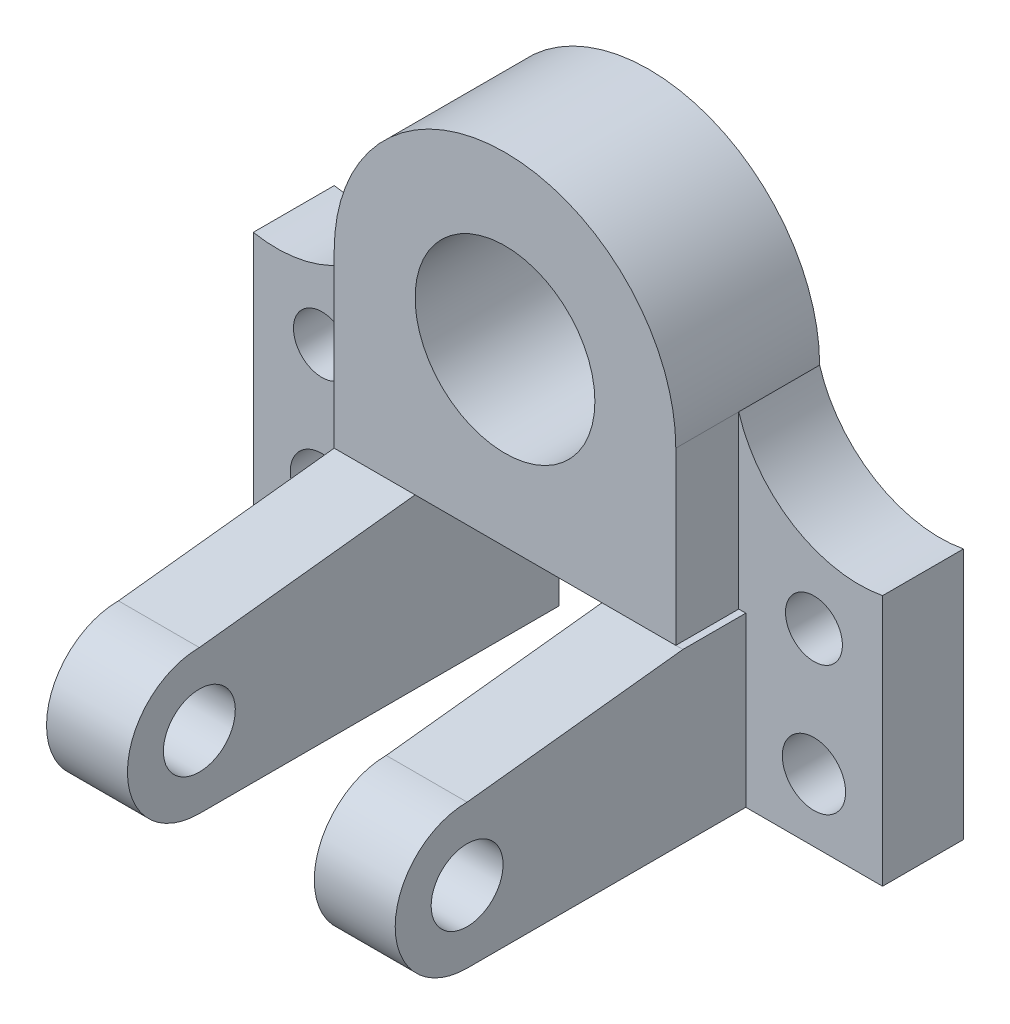
ISO-10303-21;
HEADER;
FILE_DESCRIPTION(('STEP AP214'),'2;1');
FILE_NAME('part.step','',(''),(''),'','','');
FILE_SCHEMA(('AUTOMOTIVE_DESIGN { 1 0 10303 214 1 1 1 1 }'));
ENDSEC;
DATA;
#1=APPLICATION_CONTEXT('core data for automotive mechanical design processes');
#2=APPLICATION_PROTOCOL_DEFINITION('international standard','automotive_design',2000,#1);
#3=PRODUCT_CONTEXT('',#1,'mechanical');
#4=PRODUCT('Part','Part','',(#3));
#5=PRODUCT_RELATED_PRODUCT_CATEGORY('part','',(#4));
#6=PRODUCT_DEFINITION_FORMATION('','',#4);
#7=PRODUCT_DEFINITION_CONTEXT('part definition',#1,'design');
#8=PRODUCT_DEFINITION('design','',#6,#7);
#9=PRODUCT_DEFINITION_SHAPE('','',#8);
#10=(LENGTH_UNIT() NAMED_UNIT(*) SI_UNIT(.MILLI.,.METRE.));
#11=(NAMED_UNIT(*) PLANE_ANGLE_UNIT() SI_UNIT($,.RADIAN.));
#12=(NAMED_UNIT(*) SI_UNIT($,.STERADIAN.) SOLID_ANGLE_UNIT());
#13=UNCERTAINTY_MEASURE_WITH_UNIT(LENGTH_MEASURE(1.E-05),#10,'distance_accuracy_value','');
#14=(GEOMETRIC_REPRESENTATION_CONTEXT(3) GLOBAL_UNCERTAINTY_ASSIGNED_CONTEXT((#13)) GLOBAL_UNIT_ASSIGNED_CONTEXT((#10,
#11,#12)) REPRESENTATION_CONTEXT('',''));
#15=CARTESIAN_POINT('',(0.,0.,0.));
#16=DIRECTION('',(0.,0.,1.));
#17=DIRECTION('',(1.,0.,0.));
#18=AXIS2_PLACEMENT_3D('',#15,#16,#17);
#19=CARTESIAN_POINT('',(-38.,0.,32.));
#20=DIRECTION('',(-1.,0.,0.));
#21=DIRECTION('',(0.,0.,1.));
#22=AXIS2_PLACEMENT_3D('',#19,#20,#21);
#23=PLANE('',#22);
#24=CARTESIAN_POINT('',(-38.,-59.4133546374379,80.));
#25=DIRECTION('',(-1.,0.,0.));
#26=DIRECTION('',(0.,0.,1.));
#27=AXIS2_PLACEMENT_3D('',#24,#25,#26);
#28=CIRCLE('',#27,8.);
#29=CARTESIAN_POINT('',(-38.,-59.4133546374379,88.));
#30=VERTEX_POINT('',#29);
#31=EDGE_CURVE('E434',#30,#30,#28,.T.);
#32=ORIENTED_EDGE('',*,*,#31,.F.);
#33=EDGE_LOOP('',(#32));
#34=FACE_BOUND('',#33,.T.);
#35=DIRECTION('',(0.,0.,-1.));
#36=VECTOR('',#35,1.);
#37=CARTESIAN_POINT('',(-38.,-75.4133546374379,96.));
#38=LINE('',#37,#36);
#39=CARTESIAN_POINT('',(-38.,-75.4133546374379,80.));
#40=VERTEX_POINT('',#39);
#41=CARTESIAN_POINT('',(-38.,-75.4133546374379,18.));
#42=VERTEX_POINT('',#41);
#43=EDGE_CURVE('E230',#40,#42,#38,.T.);
#44=ORIENTED_EDGE('',*,*,#43,.F.);
#45=CARTESIAN_POINT('',(-38.,-59.4133546374379,80.));
#46=DIRECTION('',(-1.,0.,0.));
#47=DIRECTION('',(0.,0.,1.));
#48=AXIS2_PLACEMENT_3D('',#45,#46,#47);
#49=CIRCLE('',#48,16.);
#50=CARTESIAN_POINT('',(-38.,-43.4133546374379,80.));
#51=VERTEX_POINT('',#50);
#52=EDGE_CURVE('E213',#40,#51,#49,.T.);
#53=ORIENTED_EDGE('',*,*,#52,.T.);
#54=DIRECTION('',(0.,0.112067782494009,-0.993700564620387));
#55=VECTOR('',#54,1.);
#56=CARTESIAN_POINT('',(-38.,-33.9591726611396,-3.82985510018196));
#57=LINE('',#56,#55);
#58=CARTESIAN_POINT('',(-38.,-38.,32.));
#59=VERTEX_POINT('',#58);
#60=EDGE_CURVE('E221',#51,#59,#57,.T.);
#61=ORIENTED_EDGE('',*,*,#60,.T.);
#62=DIRECTION('',(0.,1.,0.));
#63=VECTOR('',#62,1.);
#64=CARTESIAN_POINT('',(-38.,0.,32.));
#65=LINE('',#64,#63);
#66=CARTESIAN_POINT('',(-38.,0.,32.));
#67=VERTEX_POINT('',#66);
#68=EDGE_CURVE('E327',#59,#67,#65,.T.);
#69=ORIENTED_EDGE('',*,*,#68,.T.);
#70=DIRECTION('',(0.,0.,-1.));
#71=VECTOR('',#70,1.);
#72=CARTESIAN_POINT('',(-38.,0.,32.));
#73=LINE('',#72,#71);
#74=CARTESIAN_POINT('',(-38.,0.,18.));
#75=VERTEX_POINT('',#74);
#76=EDGE_CURVE('E345',#67,#75,#73,.T.);
#77=ORIENTED_EDGE('',*,*,#76,.T.);
#78=DIRECTION('',(0.,1.,0.));
#79=VECTOR('',#78,1.);
#80=CARTESIAN_POINT('',(-38.,0.,18.));
#81=LINE('',#80,#79);
#82=EDGE_CURVE('E240',#42,#75,#81,.T.);
#83=ORIENTED_EDGE('',*,*,#82,.F.);
#84=EDGE_LOOP('',(#44,#53,#61,#69,#77,#83));
#85=FACE_BOUND('',#84,.T.);
#86=ADVANCED_FACE('F90',(#34,#85),#23,.T.);
#87=CARTESIAN_POINT('',(-20.,-38.,96.));
#88=DIRECTION('',(-1.,0.,0.));
#89=DIRECTION('',(0.,-1.,0.));
#90=AXIS2_PLACEMENT_3D('',#87,#88,#89);
#91=PLANE('',#90);
#92=CARTESIAN_POINT('',(-20.,-59.4133546374379,80.));
#93=DIRECTION('',(-1.,0.,0.));
#94=DIRECTION('',(0.,-1.,0.));
#95=AXIS2_PLACEMENT_3D('',#92,#93,#94);
#96=CIRCLE('',#95,8.);
#97=CARTESIAN_POINT('',(-20.,-67.4133546374379,80.));
#98=VERTEX_POINT('',#97);
#99=EDGE_CURVE('E351',#98,#98,#96,.T.);
#100=ORIENTED_EDGE('',*,*,#99,.T.);
#101=EDGE_LOOP('',(#100));
#102=FACE_BOUND('',#101,.T.);
#103=CARTESIAN_POINT('',(-20.,-59.4133546374379,80.));
#104=DIRECTION('',(-1.,0.,0.));
#105=DIRECTION('',(0.,-1.,0.));
#106=AXIS2_PLACEMENT_3D('',#103,#104,#105);
#107=CIRCLE('',#106,16.);
#108=CARTESIAN_POINT('',(-20.,-75.4133546374379,80.));
#109=VERTEX_POINT('',#108);
#110=CARTESIAN_POINT('',(-20.,-43.4133546374379,80.));
#111=VERTEX_POINT('',#110);
#112=EDGE_CURVE('E350',#109,#111,#107,.T.);
#113=ORIENTED_EDGE('',*,*,#112,.F.);
#114=DIRECTION('',(0.,0.,-1.));
#115=VECTOR('',#114,1.);
#116=CARTESIAN_POINT('',(-20.,-75.4133546374379,96.));
#117=LINE('',#116,#115);
#118=CARTESIAN_POINT('',(-20.,-75.4133546374379,0.));
#119=VERTEX_POINT('',#118);
#120=EDGE_CURVE('E233',#109,#119,#117,.T.);
#121=ORIENTED_EDGE('',*,*,#120,.T.);
#122=DIRECTION('',(0.,1.,0.));
#123=VECTOR('',#122,1.);
#124=CARTESIAN_POINT('',(-20.,-38.,0.));
#125=LINE('',#124,#123);
#126=CARTESIAN_POINT('',(-20.,-38.,0.));
#127=VERTEX_POINT('',#126);
#128=EDGE_CURVE('E385',#119,#127,#125,.T.);
#129=ORIENTED_EDGE('',*,*,#128,.T.);
#130=DIRECTION('',(0.,0.,-1.));
#131=VECTOR('',#130,1.);
#132=CARTESIAN_POINT('',(-20.,-38.,96.));
#133=LINE('',#132,#131);
#134=CARTESIAN_POINT('',(-20.,-38.,32.));
#135=VERTEX_POINT('',#134);
#136=EDGE_CURVE('E244',#135,#127,#133,.T.);
#137=ORIENTED_EDGE('',*,*,#136,.F.);
#138=DIRECTION('',(0.,0.112067782494009,-0.993700564620387));
#139=VECTOR('',#138,1.);
#140=CARTESIAN_POINT('',(-20.,-45.1271563993633,95.19621197612));
#141=LINE('',#140,#139);
#142=EDGE_CURVE('E361',#111,#135,#141,.T.);
#143=ORIENTED_EDGE('',*,*,#142,.F.);
#144=EDGE_LOOP('',(#113,#121,#129,#137,#143));
#145=FACE_BOUND('',#144,.T.);
#146=ADVANCED_FACE('F392',(#102,#145),#91,.F.);
#147=CARTESIAN_POINT('',(39.5715731247638,-38.,96.));
#148=DIRECTION('',(-1.,0.,0.));
#149=DIRECTION('',(0.,0.,1.));
#150=AXIS2_PLACEMENT_3D('',#147,#148,#149);
#151=PLANE('',#150);
#152=CARTESIAN_POINT('',(39.5715731247638,-59.4133546374379,80.));
#153=DIRECTION('',(-1.,0.,0.));
#154=DIRECTION('',(0.,0.,1.));
#155=AXIS2_PLACEMENT_3D('',#152,#153,#154);
#156=CIRCLE('',#155,8.);
#157=CARTESIAN_POINT('',(39.5715731247638,-59.4133546374379,88.));
#158=VERTEX_POINT('',#157);
#159=EDGE_CURVE('E347',#158,#158,#156,.T.);
#160=ORIENTED_EDGE('',*,*,#159,.T.);
#161=EDGE_LOOP('',(#160));
#162=FACE_BOUND('',#161,.T.);
#163=CARTESIAN_POINT('',(39.5715731247638,-59.4133546374379,80.));
#164=DIRECTION('',(-1.,0.,0.));
#165=DIRECTION('',(0.,0.,1.));
#166=AXIS2_PLACEMENT_3D('',#163,#164,#165);
#167=CIRCLE('',#166,16.);
#168=CARTESIAN_POINT('',(39.5715731247638,-75.4133546374379,80.));
#169=VERTEX_POINT('',#168);
#170=CARTESIAN_POINT('',(39.5715731247638,-43.4133546374379,80.));
#171=VERTEX_POINT('',#170);
#172=EDGE_CURVE('E354',#169,#171,#167,.T.);
#173=ORIENTED_EDGE('',*,*,#172,.F.);
#174=DIRECTION('',(0.,0.,-1.));
#175=VECTOR('',#174,1.);
#176=CARTESIAN_POINT('',(39.5715731247638,-75.4133546374379,96.));
#177=LINE('',#176,#175);
#178=CARTESIAN_POINT('',(39.5715731247638,-75.4133546374379,18.));
#179=VERTEX_POINT('',#178);
#180=EDGE_CURVE('E366',#169,#179,#177,.T.);
#181=ORIENTED_EDGE('',*,*,#180,.T.);
#182=DIRECTION('',(0.,-1.,0.));
#183=VECTOR('',#182,1.);
#184=CARTESIAN_POINT('',(39.5715731247638,8.10007584438996,18.));
#185=LINE('',#184,#183);
#186=CARTESIAN_POINT('',(39.5715731247638,-38.,18.));
#187=VERTEX_POINT('',#186);
#188=EDGE_CURVE('E377',#187,#179,#185,.T.);
#189=ORIENTED_EDGE('',*,*,#188,.F.);
#190=DIRECTION('',(0.,0.,-1.));
#191=VECTOR('',#190,1.);
#192=CARTESIAN_POINT('',(39.5715731247638,-38.,96.));
#193=LINE('',#192,#191);
#194=CARTESIAN_POINT('',(39.5715731247638,-38.,32.));
#195=VERTEX_POINT('',#194);
#196=EDGE_CURVE('E372',#195,#187,#193,.T.);
#197=ORIENTED_EDGE('',*,*,#196,.F.);
#198=DIRECTION('',(0.,0.112067782494009,-0.993700564620387));
#199=VECTOR('',#198,1.);
#200=CARTESIAN_POINT('',(39.5715731247638,-45.1271563993633,95.19621197612));
#201=LINE('',#200,#199);
#202=EDGE_CURVE('E363',#171,#195,#201,.T.);
#203=ORIENTED_EDGE('',*,*,#202,.F.);
#204=EDGE_LOOP('',(#173,#181,#189,#197,#203));
#205=FACE_BOUND('',#204,.T.);
#206=ADVANCED_FACE('F449',(#162,#205),#151,.F.);
#207=CARTESIAN_POINT('',(21.5715731247638,-38.,96.));
#208=DIRECTION('',(1.,0.,0.));
#209=DIRECTION('',(0.,0.,-1.));
#210=AXIS2_PLACEMENT_3D('',#207,#208,#209);
#211=PLANE('',#210);
#212=CARTESIAN_POINT('',(21.5715731247638,-59.4133546374379,80.));
#213=DIRECTION('',(1.,0.,0.));
#214=DIRECTION('',(0.,0.,-1.));
#215=AXIS2_PLACEMENT_3D('',#212,#213,#214);
#216=CIRCLE('',#215,8.);
#217=CARTESIAN_POINT('',(21.5715731247638,-59.4133546374379,72.));
#218=VERTEX_POINT('',#217);
#219=EDGE_CURVE('E344',#218,#218,#216,.T.);
#220=ORIENTED_EDGE('',*,*,#219,.T.);
#221=EDGE_LOOP('',(#220));
#222=FACE_BOUND('',#221,.T.);
#223=DIRECTION('',(0.,0.,-1.));
#224=VECTOR('',#223,1.);
#225=CARTESIAN_POINT('',(21.5715731247638,-75.4133546374379,96.));
#226=LINE('',#225,#224);
#227=CARTESIAN_POINT('',(21.5715731247638,-75.4133546374379,80.));
#228=VERTEX_POINT('',#227);
#229=CARTESIAN_POINT('',(21.5715731247638,-75.4133546374379,0.));
#230=VERTEX_POINT('',#229);
#231=EDGE_CURVE('E367',#228,#230,#226,.T.);
#232=ORIENTED_EDGE('',*,*,#231,.F.);
#233=CARTESIAN_POINT('',(21.5715731247638,-59.4133546374379,80.));
#234=DIRECTION('',(1.,0.,0.));
#235=DIRECTION('',(0.,0.,-1.));
#236=AXIS2_PLACEMENT_3D('',#233,#234,#235);
#237=CIRCLE('',#236,16.);
#238=CARTESIAN_POINT('',(21.5715731247638,-43.4133546374379,80.));
#239=VERTEX_POINT('',#238);
#240=EDGE_CURVE('E355',#239,#228,#237,.T.);
#241=ORIENTED_EDGE('',*,*,#240,.F.);
#242=DIRECTION('',(0.,-0.112067782494009,0.993700564620387));
#243=VECTOR('',#242,1.);
#244=CARTESIAN_POINT('',(21.5715731247638,-45.1271563993633,95.19621197612));
#245=LINE('',#244,#243);
#246=CARTESIAN_POINT('',(21.5715731247638,-38.,32.));
#247=VERTEX_POINT('',#246);
#248=EDGE_CURVE('E12',#247,#239,#245,.T.);
#249=ORIENTED_EDGE('',*,*,#248,.F.);
#250=DIRECTION('',(0.,0.,-1.));
#251=VECTOR('',#250,1.);
#252=CARTESIAN_POINT('',(21.5715731247638,-38.,96.));
#253=LINE('',#252,#251);
#254=CARTESIAN_POINT('',(21.5715731247638,-38.,0.));
#255=VERTEX_POINT('',#254);
#256=EDGE_CURVE('E375',#247,#255,#253,.T.);
#257=ORIENTED_EDGE('',*,*,#256,.T.);
#258=DIRECTION('',(0.,-1.,0.));
#259=VECTOR('',#258,1.);
#260=CARTESIAN_POINT('',(21.5715731247638,-38.,0.));
#261=LINE('',#260,#259);
#262=EDGE_CURVE('E364',#255,#230,#261,.T.);
#263=ORIENTED_EDGE('',*,*,#262,.T.);
#264=EDGE_LOOP('',(#232,#241,#249,#257,#263));
#265=FACE_BOUND('',#264,.T.);
#266=ADVANCED_FACE('F420',(#222,#265),#211,.F.);
#267=CARTESIAN_POINT('',(39.5715731247638,-38.,96.));
#268=DIRECTION('',(0.,-1.,0.));
#269=DIRECTION('',(0.,0.,-1.));
#270=AXIS2_PLACEMENT_3D('',#267,#268,#269);
#271=PLANE('',#270);
#272=DIRECTION('',(-1.,0.,0.));
#273=VECTOR('',#272,1.);
#274=CARTESIAN_POINT('',(70.,-38.,32.));
#275=LINE('',#274,#273);
#276=CARTESIAN_POINT('',(38.,-38.,32.));
#277=VERTEX_POINT('',#276);
#278=EDGE_CURVE('E427',#195,#277,#275,.T.);
#279=ORIENTED_EDGE('',*,*,#278,.F.);
#280=ORIENTED_EDGE('',*,*,#196,.T.);
#281=DIRECTION('',(1.,0.,0.));
#282=VECTOR('',#281,1.);
#283=CARTESIAN_POINT('',(64.8027754405235,-38.,18.));
#284=LINE('',#283,#282);
#285=CARTESIAN_POINT('',(38.,-38.,18.));
#286=VERTEX_POINT('',#285);
#287=EDGE_CURVE('E376',#286,#187,#284,.T.);
#288=ORIENTED_EDGE('',*,*,#287,.F.);
#289=DIRECTION('',(0.,0.,-1.));
#290=VECTOR('',#289,1.);
#291=CARTESIAN_POINT('',(38.,-38.,32.));
#292=LINE('',#291,#290);
#293=EDGE_CURVE('E331',#277,#286,#292,.T.);
#294=ORIENTED_EDGE('',*,*,#293,.F.);
#295=EDGE_LOOP('',(#279,#280,#288,#294));
#296=FACE_BOUND('',#295,.T.);
#297=ADVANCED_FACE('F457',(#296),#271,.F.);
#298=CARTESIAN_POINT('',(0.,-38.,32.));
#299=DIRECTION('',(0.,-1.,0.));
#300=DIRECTION('',(0.,0.,-1.));
#301=AXIS2_PLACEMENT_3D('',#298,#299,#300);
#302=PLANE('',#301);
#303=DIRECTION('',(-1.,0.,0.));
#304=VECTOR('',#303,1.);
#305=CARTESIAN_POINT('',(0.,-38.,0.));
#306=LINE('',#305,#304);
#307=EDGE_CURVE('E102',#255,#127,#306,.T.);
#308=ORIENTED_EDGE('',*,*,#307,.F.);
#309=ORIENTED_EDGE('',*,*,#256,.F.);
#310=DIRECTION('',(-1.,0.,0.));
#311=VECTOR('',#310,1.);
#312=CARTESIAN_POINT('',(0.,-38.,32.));
#313=LINE('',#312,#311);
#314=EDGE_CURVE('E332',#247,#135,#313,.T.);
#315=ORIENTED_EDGE('',*,*,#314,.T.);
#316=ORIENTED_EDGE('',*,*,#136,.T.);
#317=EDGE_LOOP('',(#308,#309,#315,#316));
#318=FACE_BOUND('',#317,.T.);
#319=ADVANCED_FACE('F390',(#318),#302,.T.);
#320=CARTESIAN_POINT('',(64.8027754405235,8.10007584438996,18.));
#321=DIRECTION('',(0.,0.,1.));
#322=DIRECTION('',(-1.,0.,0.));
#323=AXIS2_PLACEMENT_3D('',#320,#321,#322);
#324=PLANE('',#323);
#325=CARTESIAN_POINT('',(54.7345513248247,-33.4133546374379,18.));
#326=DIRECTION('',(0.,0.,-1.));
#327=DIRECTION('',(-1.,0.,0.));
#328=AXIS2_PLACEMENT_3D('',#325,#326,#327);
#329=CIRCLE('',#328,6.33212947374812);
#330=CARTESIAN_POINT('',(48.4024218510766,-33.4133546374379,18.));
#331=VERTEX_POINT('',#330);
#332=EDGE_CURVE('E251',#331,#331,#329,.T.);
#333=ORIENTED_EDGE('',*,*,#332,.T.);
#334=EDGE_LOOP('',(#333));
#335=FACE_BOUND('',#334,.T.);
#336=CARTESIAN_POINT('',(54.7345513248247,-61.4133546374379,18.));
#337=DIRECTION('',(0.,0.,-1.));
#338=DIRECTION('',(-1.,0.,0.));
#339=AXIS2_PLACEMENT_3D('',#336,#337,#338);
#340=CIRCLE('',#339,7.04009535410836);
#341=CARTESIAN_POINT('',(47.6944559707163,-61.4133546374379,18.));
#342=VERTEX_POINT('',#341);
#343=EDGE_CURVE('E250',#342,#342,#340,.T.);
#344=ORIENTED_EDGE('',*,*,#343,.T.);
#345=EDGE_LOOP('',(#344));
#346=FACE_BOUND('',#345,.T.);
#347=ORIENTED_EDGE('',*,*,#287,.T.);
#348=ORIENTED_EDGE('',*,*,#188,.T.);
#349=DIRECTION('',(-1.,0.,0.));
#350=VECTOR('',#349,1.);
#351=CARTESIAN_POINT('',(38.,-75.4133546374379,18.));
#352=LINE('',#351,#350);
#353=CARTESIAN_POINT('',(70.,-75.4133546374379,18.));
#354=VERTEX_POINT('',#353);
#355=EDGE_CURVE('E266',#354,#179,#352,.T.);
#356=ORIENTED_EDGE('',*,*,#355,.F.);
#357=DIRECTION('',(0.,-1.,0.));
#358=VECTOR('',#357,1.);
#359=CARTESIAN_POINT('',(70.,-75.4133546374379,18.));
#360=LINE('',#359,#358);
#361=CARTESIAN_POINT('',(70.,-19.4133546374379,18.));
#362=VERTEX_POINT('',#361);
#363=EDGE_CURVE('E265',#362,#354,#360,.T.);
#364=ORIENTED_EDGE('',*,*,#363,.F.);
#365=CARTESIAN_POINT('',(64.8027754405235,8.10007584438996,18.));
#366=DIRECTION('',(0.,0.,1.));
#367=DIRECTION('',(-1.,0.,0.));
#368=AXIS2_PLACEMENT_3D('',#365,#366,#367);
#369=CIRCLE('',#368,28.);
#370=CARTESIAN_POINT('',(38.,0.,18.));
#371=VERTEX_POINT('',#370);
#372=EDGE_CURVE('E259',#371,#362,#369,.T.);
#373=ORIENTED_EDGE('',*,*,#372,.F.);
#374=DIRECTION('',(0.,1.,0.));
#375=VECTOR('',#374,1.);
#376=CARTESIAN_POINT('',(38.,0.,18.));
#377=LINE('',#376,#375);
#378=EDGE_CURVE('E115',#286,#371,#377,.T.);
#379=ORIENTED_EDGE('',*,*,#378,.F.);
#380=EDGE_LOOP('',(#347,#348,#356,#364,#373,#379));
#381=FACE_BOUND('',#380,.T.);
#382=ADVANCED_FACE('F455',(#335,#346,#381),#324,.T.);
#383=CARTESIAN_POINT('',(38.,0.,32.));
#384=DIRECTION('',(1.,0.,0.));
#385=DIRECTION('',(0.,0.,-1.));
#386=AXIS2_PLACEMENT_3D('',#383,#384,#385);
#387=PLANE('',#386);
#388=ORIENTED_EDGE('',*,*,#378,.T.);
#389=DIRECTION('',(0.,0.,-1.));
#390=VECTOR('',#389,1.);
#391=CARTESIAN_POINT('',(38.,0.,32.));
#392=LINE('',#391,#390);
#393=CARTESIAN_POINT('',(38.,0.,32.));
#394=VERTEX_POINT('',#393);
#395=EDGE_CURVE('E100',#394,#371,#392,.T.);
#396=ORIENTED_EDGE('',*,*,#395,.F.);
#397=DIRECTION('',(0.,-1.,0.));
#398=VECTOR('',#397,1.);
#399=CARTESIAN_POINT('',(38.,0.,32.));
#400=LINE('',#399,#398);
#401=EDGE_CURVE('E323',#394,#277,#400,.T.);
#402=ORIENTED_EDGE('',*,*,#401,.T.);
#403=ORIENTED_EDGE('',*,*,#293,.T.);
#404=EDGE_LOOP('',(#388,#396,#402,#403));
#405=FACE_BOUND('',#404,.T.);
#406=ADVANCED_FACE('F460',(#405),#387,.T.);
#407=CARTESIAN_POINT('',(0.,0.,32.));
#408=DIRECTION('',(0.,0.,-1.));
#409=DIRECTION('',(-1.,0.,0.));
#410=AXIS2_PLACEMENT_3D('',#407,#408,#409);
#411=CYLINDRICAL_SURFACE('',#410,38.);
#412=CARTESIAN_POINT('',(0.,0.,0.));
#413=DIRECTION('',(0.,0.,1.));
#414=DIRECTION('',(1.,0.,0.));
#415=AXIS2_PLACEMENT_3D('',#412,#413,#414);
#416=CIRCLE('',#415,38.);
#417=CARTESIAN_POINT('',(38.,0.,0.));
#418=VERTEX_POINT('',#417);
#419=CARTESIAN_POINT('',(-38.,0.,0.));
#420=VERTEX_POINT('',#419);
#421=EDGE_CURVE('E337',#418,#420,#416,.T.);
#422=ORIENTED_EDGE('',*,*,#421,.T.);
#423=DIRECTION('',(0.,0.,-1.));
#424=VECTOR('',#423,1.);
#425=CARTESIAN_POINT('',(-38.,0.,18.));
#426=LINE('',#425,#424);
#427=EDGE_CURVE('E301',#75,#420,#426,.T.);
#428=ORIENTED_EDGE('',*,*,#427,.F.);
#429=ORIENTED_EDGE('',*,*,#76,.F.);
#430=CARTESIAN_POINT('',(0.,0.,32.));
#431=DIRECTION('',(0.,0.,1.));
#432=DIRECTION('',(1.,0.,0.));
#433=AXIS2_PLACEMENT_3D('',#430,#431,#432);
#434=CIRCLE('',#433,38.);
#435=EDGE_CURVE('E326',#394,#67,#434,.T.);
#436=ORIENTED_EDGE('',*,*,#435,.F.);
#437=ORIENTED_EDGE('',*,*,#395,.T.);
#438=DIRECTION('',(0.,0.,-1.));
#439=VECTOR('',#438,1.);
#440=CARTESIAN_POINT('',(38.,0.,18.));
#441=LINE('',#440,#439);
#442=EDGE_CURVE('E269',#371,#418,#441,.T.);
#443=ORIENTED_EDGE('',*,*,#442,.T.);
#444=EDGE_LOOP('',(#422,#428,#429,#436,#437,#443));
#445=FACE_BOUND('',#444,.T.);
#446=ADVANCED_FACE('F458',(#445),#411,.T.);
#447=CARTESIAN_POINT('',(0.,0.,32.));
#448=DIRECTION('',(0.,0.,-1.));
#449=DIRECTION('',(-1.,0.,0.));
#450=AXIS2_PLACEMENT_3D('',#447,#448,#449);
#451=CYLINDRICAL_SURFACE('',#450,20.);
#452=CARTESIAN_POINT('',(0.,0.,32.));
#453=DIRECTION('',(0.,0.,1.));
#454=DIRECTION('',(1.,0.,0.));
#455=AXIS2_PLACEMENT_3D('',#452,#453,#454);
#456=CIRCLE('',#455,20.);
#457=CARTESIAN_POINT('',(20.,0.,32.));
#458=VERTEX_POINT('',#457);
#459=EDGE_CURVE('E319',#458,#458,#456,.T.);
#460=ORIENTED_EDGE('',*,*,#459,.T.);
#461=EDGE_LOOP('',(#460));
#462=FACE_BOUND('',#461,.T.);
#463=CARTESIAN_POINT('',(0.,0.,0.));
#464=DIRECTION('',(0.,0.,1.));
#465=DIRECTION('',(1.,0.,0.));
#466=AXIS2_PLACEMENT_3D('',#463,#464,#465);
#467=CIRCLE('',#466,20.);
#468=CARTESIAN_POINT('',(20.,0.,0.));
#469=VERTEX_POINT('',#468);
#470=EDGE_CURVE('E317',#469,#469,#467,.T.);
#471=ORIENTED_EDGE('',*,*,#470,.F.);
#472=EDGE_LOOP('',(#471));
#473=FACE_BOUND('',#472,.T.);
#474=ADVANCED_FACE('F93',(#462,#473),#451,.F.);
#475=CARTESIAN_POINT('',(0.,0.,32.));
#476=DIRECTION('',(0.,0.,1.));
#477=DIRECTION('',(1.,0.,0.));
#478=AXIS2_PLACEMENT_3D('',#475,#476,#477);
#479=PLANE('',#478);
#480=ORIENTED_EDGE('',*,*,#459,.F.);
#481=EDGE_LOOP('',(#480));
#482=FACE_BOUND('',#481,.T.);
#483=ORIENTED_EDGE('',*,*,#401,.F.);
#484=ORIENTED_EDGE('',*,*,#435,.T.);
#485=ORIENTED_EDGE('',*,*,#68,.F.);
#486=DIRECTION('',(1.,0.,0.));
#487=VECTOR('',#486,1.);
#488=CARTESIAN_POINT('',(0.,-38.,32.));
#489=LINE('',#488,#487);
#490=EDGE_CURVE('E236',#59,#135,#489,.T.);
#491=ORIENTED_EDGE('',*,*,#490,.T.);
#492=ORIENTED_EDGE('',*,*,#314,.F.);
#493=EDGE_CURVE('E335',#277,#247,#313,.T.);
#494=ORIENTED_EDGE('',*,*,#493,.F.);
#495=EDGE_LOOP('',(#483,#484,#485,#491,#492,#494));
#496=FACE_BOUND('',#495,.T.);
#497=ADVANCED_FACE('F422',(#482,#496),#479,.T.);
#498=CARTESIAN_POINT('',(0.,0.,0.));
#499=DIRECTION('',(0.,0.,1.));
#500=DIRECTION('',(1.,0.,0.));
#501=AXIS2_PLACEMENT_3D('',#498,#499,#500);
#502=PLANE('',#501);
#503=DIRECTION('',(-1.,0.,0.));
#504=VECTOR('',#503,1.);
#505=CARTESIAN_POINT('',(38.,-75.4133546374379,0.));
#506=LINE('',#505,#504);
#507=CARTESIAN_POINT('',(70.,-75.4133546374379,0.));
#508=VERTEX_POINT('',#507);
#509=EDGE_CURVE('E263',#508,#230,#506,.T.);
#510=ORIENTED_EDGE('',*,*,#509,.T.);
#511=ORIENTED_EDGE('',*,*,#262,.F.);
#512=ORIENTED_EDGE('',*,*,#307,.T.);
#513=ORIENTED_EDGE('',*,*,#128,.F.);
#514=DIRECTION('',(1.,0.,0.));
#515=VECTOR('',#514,1.);
#516=CARTESIAN_POINT('',(-38.,-75.4133546374379,0.));
#517=LINE('',#516,#515);
#518=CARTESIAN_POINT('',(-70.,-75.4133546374379,0.));
#519=VERTEX_POINT('',#518);
#520=EDGE_CURVE('E300',#519,#119,#517,.T.);
#521=ORIENTED_EDGE('',*,*,#520,.F.);
#522=DIRECTION('',(0.,-1.,0.));
#523=VECTOR('',#522,1.);
#524=CARTESIAN_POINT('',(-70.,-75.4133546374379,0.));
#525=LINE('',#524,#523);
#526=CARTESIAN_POINT('',(-70.,-19.4133546374379,0.));
#527=VERTEX_POINT('',#526);
#528=EDGE_CURVE('E306',#527,#519,#525,.T.);
#529=ORIENTED_EDGE('',*,*,#528,.F.);
#530=CARTESIAN_POINT('',(-64.8027754405235,8.10007584438996,0.));
#531=DIRECTION('',(0.,0.,-1.));
#532=DIRECTION('',(1.,0.,0.));
#533=AXIS2_PLACEMENT_3D('',#530,#531,#532);
#534=CIRCLE('',#533,28.);
#535=EDGE_CURVE('E291',#420,#527,#534,.T.);
#536=ORIENTED_EDGE('',*,*,#535,.F.);
#537=ORIENTED_EDGE('',*,*,#421,.F.);
#538=CARTESIAN_POINT('',(64.8027754405235,8.10007584438996,0.));
#539=DIRECTION('',(0.,0.,1.));
#540=DIRECTION('',(-1.,0.,0.));
#541=AXIS2_PLACEMENT_3D('',#538,#539,#540);
#542=CIRCLE('',#541,28.);
#543=CARTESIAN_POINT('',(70.,-19.4133546374379,0.));
#544=VERTEX_POINT('',#543);
#545=EDGE_CURVE('E258',#418,#544,#542,.T.);
#546=ORIENTED_EDGE('',*,*,#545,.T.);
#547=DIRECTION('',(0.,-1.,0.));
#548=VECTOR('',#547,1.);
#549=CARTESIAN_POINT('',(70.,-75.4133546374379,0.));
#550=LINE('',#549,#548);
#551=EDGE_CURVE('E272',#544,#508,#550,.T.);
#552=ORIENTED_EDGE('',*,*,#551,.T.);
#553=EDGE_LOOP('',(#510,#511,#512,#513,#521,#529,#536,#537,#546,#552));
#554=FACE_BOUND('',#553,.T.);
#555=CARTESIAN_POINT('',(54.7345513248247,-61.4133546374379,0.));
#556=DIRECTION('',(0.,0.,-1.));
#557=DIRECTION('',(-1.,0.,0.));
#558=AXIS2_PLACEMENT_3D('',#555,#556,#557);
#559=CIRCLE('',#558,7.04009535410836);
#560=CARTESIAN_POINT('',(47.6944559707163,-61.4133546374379,0.));
#561=VERTEX_POINT('',#560);
#562=EDGE_CURVE('E241',#561,#561,#559,.T.);
#563=ORIENTED_EDGE('',*,*,#562,.F.);
#564=EDGE_LOOP('',(#563));
#565=FACE_BOUND('',#564,.T.);
#566=CARTESIAN_POINT('',(54.7345513248247,-33.4133546374379,0.));
#567=DIRECTION('',(0.,0.,-1.));
#568=DIRECTION('',(-1.,0.,0.));
#569=AXIS2_PLACEMENT_3D('',#566,#567,#568);
#570=CIRCLE('',#569,6.33212947374812);
#571=CARTESIAN_POINT('',(48.4024218510766,-33.4133546374379,0.));
#572=VERTEX_POINT('',#571);
#573=EDGE_CURVE('E246',#572,#572,#570,.T.);
#574=ORIENTED_EDGE('',*,*,#573,.F.);
#575=EDGE_LOOP('',(#574));
#576=FACE_BOUND('',#575,.T.);
#577=ORIENTED_EDGE('',*,*,#470,.T.);
#578=EDGE_LOOP('',(#577));
#579=FACE_BOUND('',#578,.T.);
#580=CARTESIAN_POINT('',(-54.7345513248247,-61.4133546374379,0.));
#581=DIRECTION('',(0.,0.,1.));
#582=DIRECTION('',(1.,0.,0.));
#583=AXIS2_PLACEMENT_3D('',#580,#581,#582);
#584=CIRCLE('',#583,7.04009535410836);
#585=CARTESIAN_POINT('',(-47.6944559707163,-61.4133546374379,0.));
#586=VERTEX_POINT('',#585);
#587=EDGE_CURVE('E284',#586,#586,#584,.T.);
#588=ORIENTED_EDGE('',*,*,#587,.T.);
#589=EDGE_LOOP('',(#588));
#590=FACE_BOUND('',#589,.T.);
#591=CARTESIAN_POINT('',(-54.7345513248247,-33.4133546374379,0.));
#592=DIRECTION('',(0.,0.,1.));
#593=DIRECTION('',(1.,0.,0.));
#594=AXIS2_PLACEMENT_3D('',#591,#592,#593);
#595=CIRCLE('',#594,6.33212947374812);
#596=CARTESIAN_POINT('',(-48.4024218510766,-33.4133546374379,0.));
#597=VERTEX_POINT('',#596);
#598=EDGE_CURVE('E290',#597,#597,#595,.T.);
#599=ORIENTED_EDGE('',*,*,#598,.T.);
#600=EDGE_LOOP('',(#599));
#601=FACE_BOUND('',#600,.T.);
#602=ADVANCED_FACE('F393',(#554,#565,#576,#579,#590,#601),#502,.F.);
#603=CARTESIAN_POINT('',(-64.8027754405235,8.10007584438996,18.));
#604=DIRECTION('',(0.,0.,1.));
#605=DIRECTION('',(1.,0.,0.));
#606=AXIS2_PLACEMENT_3D('',#603,#604,#605);
#607=PLANE('',#606);
#608=CARTESIAN_POINT('',(-54.7345513248247,-33.4133546374379,18.));
#609=DIRECTION('',(0.,0.,1.));
#610=DIRECTION('',(1.,0.,0.));
#611=AXIS2_PLACEMENT_3D('',#608,#609,#610);
#612=CIRCLE('',#611,6.33212947374812);
#613=CARTESIAN_POINT('',(-48.4024218510766,-33.4133546374379,18.));
#614=VERTEX_POINT('',#613);
#615=EDGE_CURVE('E286',#614,#614,#612,.T.);
#616=ORIENTED_EDGE('',*,*,#615,.F.);
#617=EDGE_LOOP('',(#616));
#618=FACE_BOUND('',#617,.T.);
#619=CARTESIAN_POINT('',(-64.8027754405235,8.10007584438996,18.));
#620=DIRECTION('',(0.,0.,-1.));
#621=DIRECTION('',(1.,0.,0.));
#622=AXIS2_PLACEMENT_3D('',#619,#620,#621);
#623=CIRCLE('',#622,28.);
#624=CARTESIAN_POINT('',(-70.,-19.4133546374379,18.));
#625=VERTEX_POINT('',#624);
#626=EDGE_CURVE('E296',#75,#625,#623,.T.);
#627=ORIENTED_EDGE('',*,*,#626,.T.);
#628=DIRECTION('',(0.,-1.,0.));
#629=VECTOR('',#628,1.);
#630=CARTESIAN_POINT('',(-70.,-75.4133546374379,18.));
#631=LINE('',#630,#629);
#632=CARTESIAN_POINT('',(-70.,-75.4133546374379,18.));
#633=VERTEX_POINT('',#632);
#634=EDGE_CURVE('E298',#625,#633,#631,.T.);
#635=ORIENTED_EDGE('',*,*,#634,.T.);
#636=DIRECTION('',(1.,0.,0.));
#637=VECTOR('',#636,1.);
#638=CARTESIAN_POINT('',(-38.,-75.4133546374379,18.));
#639=LINE('',#638,#637);
#640=EDGE_CURVE('E305',#633,#42,#639,.T.);
#641=ORIENTED_EDGE('',*,*,#640,.T.);
#642=ORIENTED_EDGE('',*,*,#82,.T.);
#643=EDGE_LOOP('',(#627,#635,#641,#642));
#644=FACE_BOUND('',#643,.T.);
#645=CARTESIAN_POINT('',(-54.7345513248247,-61.4133546374379,18.));
#646=DIRECTION('',(0.,0.,1.));
#647=DIRECTION('',(1.,0.,0.));
#648=AXIS2_PLACEMENT_3D('',#645,#646,#647);
#649=CIRCLE('',#648,7.04009535410836);
#650=CARTESIAN_POINT('',(-47.6944559707163,-61.4133546374379,18.));
#651=VERTEX_POINT('',#650);
#652=EDGE_CURVE('E283',#651,#651,#649,.T.);
#653=ORIENTED_EDGE('',*,*,#652,.F.);
#654=EDGE_LOOP('',(#653));
#655=FACE_BOUND('',#654,.T.);
#656=ADVANCED_FACE('F484',(#618,#644,#655),#607,.T.);
#657=CARTESIAN_POINT('',(-64.8027754405235,8.10007584438996,18.));
#658=DIRECTION('',(0.,0.,-1.));
#659=DIRECTION('',(-1.,0.,0.));
#660=AXIS2_PLACEMENT_3D('',#657,#658,#659);
#661=CYLINDRICAL_SURFACE('',#660,28.);
#662=ORIENTED_EDGE('',*,*,#535,.T.);
#663=DIRECTION('',(0.,0.,-1.));
#664=VECTOR('',#663,1.);
#665=CARTESIAN_POINT('',(-70.,-19.4133546374379,18.));
#666=LINE('',#665,#664);
#667=EDGE_CURVE('E316',#625,#527,#666,.T.);
#668=ORIENTED_EDGE('',*,*,#667,.F.);
#669=ORIENTED_EDGE('',*,*,#626,.F.);
#670=ORIENTED_EDGE('',*,*,#427,.T.);
#671=EDGE_LOOP('',(#662,#668,#669,#670));
#672=FACE_BOUND('',#671,.T.);
#673=ADVANCED_FACE('F405',(#672),#661,.F.);
#674=CARTESIAN_POINT('',(-70.,-75.4133546374379,18.));
#675=DIRECTION('',(1.,0.,0.));
#676=DIRECTION('',(0.,0.,-1.));
#677=AXIS2_PLACEMENT_3D('',#674,#675,#676);
#678=PLANE('',#677);
#679=ORIENTED_EDGE('',*,*,#528,.T.);
#680=DIRECTION('',(0.,0.,-1.));
#681=VECTOR('',#680,1.);
#682=CARTESIAN_POINT('',(-70.,-75.4133546374379,18.));
#683=LINE('',#682,#681);
#684=EDGE_CURVE('E311',#633,#519,#683,.T.);
#685=ORIENTED_EDGE('',*,*,#684,.F.);
#686=ORIENTED_EDGE('',*,*,#634,.F.);
#687=ORIENTED_EDGE('',*,*,#667,.T.);
#688=EDGE_LOOP('',(#679,#685,#686,#687));
#689=FACE_BOUND('',#688,.T.);
#690=ADVANCED_FACE('F398',(#689),#678,.F.);
#691=CARTESIAN_POINT('',(-38.,-75.4133546374379,18.));
#692=DIRECTION('',(0.,1.,0.));
#693=DIRECTION('',(-1.,0.,0.));
#694=AXIS2_PLACEMENT_3D('',#691,#692,#693);
#695=PLANE('',#694);
#696=ORIENTED_EDGE('',*,*,#120,.F.);
#697=DIRECTION('',(-1.,0.,0.));
#698=VECTOR('',#697,1.);
#699=CARTESIAN_POINT('',(70.,-75.4133546374379,80.));
#700=LINE('',#699,#698);
#701=EDGE_CURVE('E216',#109,#40,#700,.T.);
#702=ORIENTED_EDGE('',*,*,#701,.T.);
#703=ORIENTED_EDGE('',*,*,#43,.T.);
#704=ORIENTED_EDGE('',*,*,#640,.F.);
#705=ORIENTED_EDGE('',*,*,#684,.T.);
#706=ORIENTED_EDGE('',*,*,#520,.T.);
#707=EDGE_LOOP('',(#696,#702,#703,#704,#705,#706));
#708=FACE_BOUND('',#707,.T.);
#709=ADVANCED_FACE('F229',(#708),#695,.F.);
#710=CARTESIAN_POINT('',(-54.7345513248247,-33.4133546374379,18.));
#711=DIRECTION('',(0.,0.,-1.));
#712=DIRECTION('',(-1.,0.,0.));
#713=AXIS2_PLACEMENT_3D('',#710,#711,#712);
#714=CYLINDRICAL_SURFACE('',#713,6.33212947374812);
#715=ORIENTED_EDGE('',*,*,#615,.T.);
#716=EDGE_LOOP('',(#715));
#717=FACE_BOUND('',#716,.T.);
#718=ORIENTED_EDGE('',*,*,#598,.F.);
#719=EDGE_LOOP('',(#718));
#720=FACE_BOUND('',#719,.T.);
#721=ADVANCED_FACE('F494',(#717,#720),#714,.F.);
#722=CARTESIAN_POINT('',(-54.7345513248247,-61.4133546374379,18.));
#723=DIRECTION('',(0.,0.,-1.));
#724=DIRECTION('',(-1.,0.,0.));
#725=AXIS2_PLACEMENT_3D('',#722,#723,#724);
#726=CYLINDRICAL_SURFACE('',#725,7.04009535410836);
#727=ORIENTED_EDGE('',*,*,#652,.T.);
#728=EDGE_LOOP('',(#727));
#729=FACE_BOUND('',#728,.T.);
#730=ORIENTED_EDGE('',*,*,#587,.F.);
#731=EDGE_LOOP('',(#730));
#732=FACE_BOUND('',#731,.T.);
#733=ADVANCED_FACE('F498',(#729,#732),#726,.F.);
#734=CARTESIAN_POINT('',(64.8027754405235,8.10007584438996,18.));
#735=DIRECTION('',(0.,0.,-1.));
#736=DIRECTION('',(1.,0.,0.));
#737=AXIS2_PLACEMENT_3D('',#734,#735,#736);
#738=CYLINDRICAL_SURFACE('',#737,28.);
#739=ORIENTED_EDGE('',*,*,#545,.F.);
#740=ORIENTED_EDGE('',*,*,#442,.F.);
#741=ORIENTED_EDGE('',*,*,#372,.T.);
#742=DIRECTION('',(0.,0.,-1.));
#743=VECTOR('',#742,1.);
#744=CARTESIAN_POINT('',(70.,-19.4133546374379,18.));
#745=LINE('',#744,#743);
#746=EDGE_CURVE('E281',#362,#544,#745,.T.);
#747=ORIENTED_EDGE('',*,*,#746,.T.);
#748=EDGE_LOOP('',(#739,#740,#741,#747));
#749=FACE_BOUND('',#748,.T.);
#750=ADVANCED_FACE('F408',(#749),#738,.F.);
#751=CARTESIAN_POINT('',(70.,-75.4133546374379,18.));
#752=DIRECTION('',(-1.,0.,0.));
#753=DIRECTION('',(0.,0.,-1.));
#754=AXIS2_PLACEMENT_3D('',#751,#752,#753);
#755=PLANE('',#754);
#756=ORIENTED_EDGE('',*,*,#551,.F.);
#757=ORIENTED_EDGE('',*,*,#746,.F.);
#758=ORIENTED_EDGE('',*,*,#363,.T.);
#759=DIRECTION('',(0.,0.,-1.));
#760=VECTOR('',#759,1.);
#761=CARTESIAN_POINT('',(70.,-75.4133546374379,18.));
#762=LINE('',#761,#760);
#763=EDGE_CURVE('E276',#354,#508,#762,.T.);
#764=ORIENTED_EDGE('',*,*,#763,.T.);
#765=EDGE_LOOP('',(#756,#757,#758,#764));
#766=FACE_BOUND('',#765,.T.);
#767=ADVANCED_FACE('F414',(#766),#755,.F.);
#768=CARTESIAN_POINT('',(38.,-75.4133546374379,18.));
#769=DIRECTION('',(0.,1.,0.));
#770=DIRECTION('',(1.,0.,0.));
#771=AXIS2_PLACEMENT_3D('',#768,#769,#770);
#772=PLANE('',#771);
#773=ORIENTED_EDGE('',*,*,#180,.F.);
#774=EDGE_CURVE('E223',#169,#228,#700,.T.);
#775=ORIENTED_EDGE('',*,*,#774,.T.);
#776=ORIENTED_EDGE('',*,*,#231,.T.);
#777=ORIENTED_EDGE('',*,*,#509,.F.);
#778=ORIENTED_EDGE('',*,*,#763,.F.);
#779=ORIENTED_EDGE('',*,*,#355,.T.);
#780=EDGE_LOOP('',(#773,#775,#776,#777,#778,#779));
#781=FACE_BOUND('',#780,.T.);
#782=ADVANCED_FACE('F441',(#781),#772,.F.);
#783=CARTESIAN_POINT('',(54.7345513248247,-33.4133546374379,18.));
#784=DIRECTION('',(0.,0.,-1.));
#785=DIRECTION('',(1.,0.,0.));
#786=AXIS2_PLACEMENT_3D('',#783,#784,#785);
#787=CYLINDRICAL_SURFACE('',#786,6.33212947374812);
#788=ORIENTED_EDGE('',*,*,#332,.F.);
#789=EDGE_LOOP('',(#788));
#790=FACE_BOUND('',#789,.T.);
#791=ORIENTED_EDGE('',*,*,#573,.T.);
#792=EDGE_LOOP('',(#791));
#793=FACE_BOUND('',#792,.T.);
#794=ADVANCED_FACE('F506',(#790,#793),#787,.F.);
#795=CARTESIAN_POINT('',(54.7345513248247,-61.4133546374379,18.));
#796=DIRECTION('',(0.,0.,-1.));
#797=DIRECTION('',(1.,0.,0.));
#798=AXIS2_PLACEMENT_3D('',#795,#796,#797);
#799=CYLINDRICAL_SURFACE('',#798,7.04009535410836);
#800=ORIENTED_EDGE('',*,*,#343,.F.);
#801=EDGE_LOOP('',(#800));
#802=FACE_BOUND('',#801,.T.);
#803=ORIENTED_EDGE('',*,*,#562,.T.);
#804=EDGE_LOOP('',(#803));
#805=FACE_BOUND('',#804,.T.);
#806=ADVANCED_FACE('F516',(#802,#805),#799,.F.);
#807=CARTESIAN_POINT('',(70.,-59.4133546374379,80.));
#808=DIRECTION('',(-1.,0.,0.));
#809=DIRECTION('',(0.,0.,1.));
#810=AXIS2_PLACEMENT_3D('',#807,#808,#809);
#811=CYLINDRICAL_SURFACE('',#810,16.);
#812=ORIENTED_EDGE('',*,*,#172,.T.);
#813=DIRECTION('',(-1.,0.,0.));
#814=VECTOR('',#813,1.);
#815=CARTESIAN_POINT('',(70.,-43.4133546374379,80.));
#816=LINE('',#815,#814);
#817=EDGE_CURVE('E433',#171,#239,#816,.T.);
#818=ORIENTED_EDGE('',*,*,#817,.T.);
#819=ORIENTED_EDGE('',*,*,#240,.T.);
#820=ORIENTED_EDGE('',*,*,#774,.F.);
#821=EDGE_LOOP('',(#812,#818,#819,#820));
#822=FACE_BOUND('',#821,.T.);
#823=ADVANCED_FACE('F442',(#822),#811,.T.);
#824=CARTESIAN_POINT('',(70.,-33.9591726611396,-3.82985510018196));
#825=DIRECTION('',(0.,0.993700564620387,0.112067782494009));
#826=DIRECTION('',(0.,-0.112067782494009,0.993700564620387));
#827=AXIS2_PLACEMENT_3D('',#824,#825,#826);
#828=PLANE('',#827);
#829=ORIENTED_EDGE('',*,*,#202,.T.);
#830=ORIENTED_EDGE('',*,*,#278,.T.);
#831=ORIENTED_EDGE('',*,*,#493,.T.);
#832=ORIENTED_EDGE('',*,*,#248,.T.);
#833=ORIENTED_EDGE('',*,*,#817,.F.);
#834=EDGE_LOOP('',(#829,#830,#831,#832,#833));
#835=FACE_BOUND('',#834,.T.);
#836=ADVANCED_FACE('F536',(#835),#828,.T.);
#837=CARTESIAN_POINT('',(70.,-59.4133546374379,80.));
#838=DIRECTION('',(-1.,0.,0.));
#839=DIRECTION('',(0.,0.,1.));
#840=AXIS2_PLACEMENT_3D('',#837,#838,#839);
#841=CYLINDRICAL_SURFACE('',#840,8.);
#842=ORIENTED_EDGE('',*,*,#219,.F.);
#843=EDGE_LOOP('',(#842));
#844=FACE_BOUND('',#843,.T.);
#845=ORIENTED_EDGE('',*,*,#159,.F.);
#846=EDGE_LOOP('',(#845));
#847=FACE_BOUND('',#846,.T.);
#848=ADVANCED_FACE('F535',(#844,#847),#841,.F.);
#849=ORIENTED_EDGE('',*,*,#142,.T.);
#850=ORIENTED_EDGE('',*,*,#490,.F.);
#851=ORIENTED_EDGE('',*,*,#60,.F.);
#852=EDGE_CURVE('E218',#111,#51,#816,.T.);
#853=ORIENTED_EDGE('',*,*,#852,.F.);
#854=EDGE_LOOP('',(#849,#850,#851,#853));
#855=FACE_BOUND('',#854,.T.);
#856=ADVANCED_FACE('F428',(#855),#828,.T.);
#857=ORIENTED_EDGE('',*,*,#112,.T.);
#858=ORIENTED_EDGE('',*,*,#852,.T.);
#859=ORIENTED_EDGE('',*,*,#52,.F.);
#860=ORIENTED_EDGE('',*,*,#701,.F.);
#861=EDGE_LOOP('',(#857,#858,#859,#860));
#862=FACE_BOUND('',#861,.T.);
#863=ADVANCED_FACE('F214',(#862),#811,.T.);
#864=ORIENTED_EDGE('',*,*,#31,.T.);
#865=EDGE_LOOP('',(#864));
#866=FACE_BOUND('',#865,.T.);
#867=ORIENTED_EDGE('',*,*,#99,.F.);
#868=EDGE_LOOP('',(#867));
#869=FACE_BOUND('',#868,.T.);
#870=ADVANCED_FACE('F526',(#866,#869),#841,.F.);
#871=CLOSED_SHELL('',(#86,#146,#206,#266,#297,#319,#382,#406,#446,#474,#497,#602,#656,#673,#690,
#709,#721,#733,#750,#767,#782,#794,#806,#823,#836,#848,#856,#863,#870));
#872=MANIFOLD_SOLID_BREP('B2',#871);
#873=ADVANCED_BREP_SHAPE_REPRESENTATION('',(#18,#872),#14);
#874=SHAPE_DEFINITION_REPRESENTATION(#9,#873);
ENDSEC;
END-ISO-10303-21;
